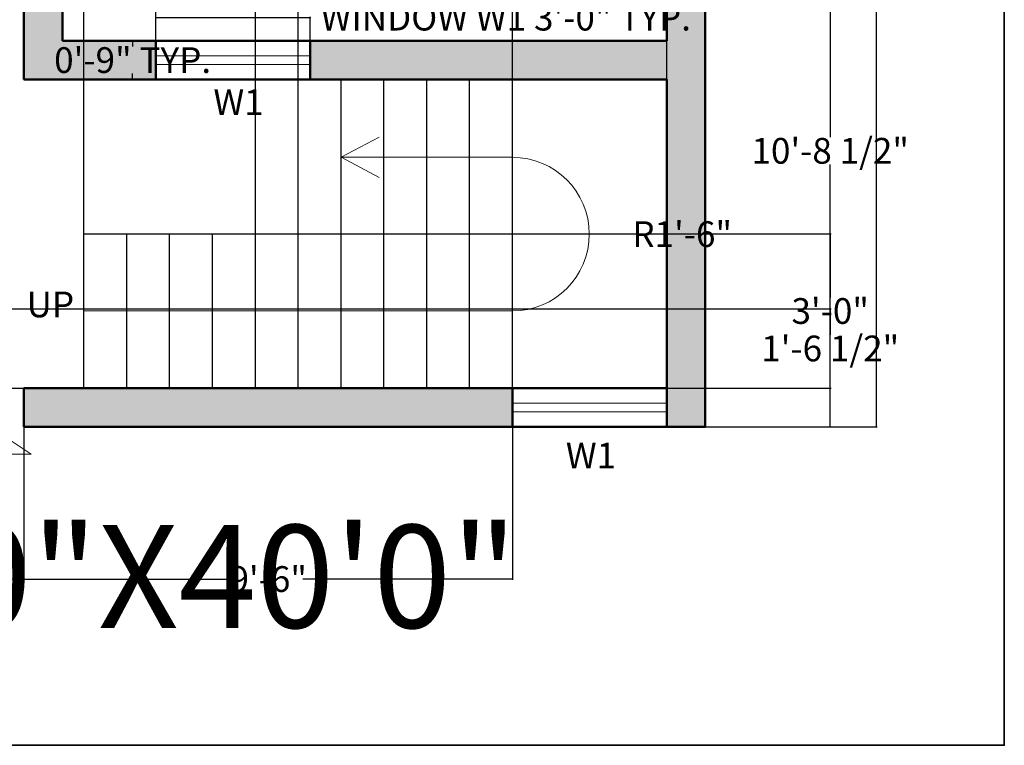
# Model space of a CAD drawing. Units: inches. Extents: x 125920 to 126336, y 366134 to 366735.
# Tile 2 of 6: x 126106 to 126336, y 366134 to 366303. Entities that reach past the tile are written whole.
import ezdxf

# ---------------------------------------------------------------- set-up
doc = ezdxf.new("R2010")
doc.units = ezdxf.units.IN
doc.header["$MEASUREMENT"] = 0
for name, color, linetype, lineweight in [('A-ANNO-DIMS', 2, 'Continuous', 18), ('A-ANNO-SYMB', 7, 'Continuous', 18), ('A-ANNO-TEXT', 7, 'Continuous', 18), ('A-ANNO-TTLB', 7, 'Continuous', 35), ('A-FLOR-STRS', 7, 'Continuous', 25), ('A-GLAZ', 4, 'Continuous', 18), ('A-WALL', 7, 'Continuous', 50)]:
    doc.layers.add(name, color=color, linetype=linetype, lineweight=lineweight)
doc.layers.add('A-WALL-PATT', color=18, linetype='Continuous', lineweight=13, true_color=0x000000)
doc.styles.get("Standard").update_dxf_attribs({"font": 'arial.ttf'})
doc.dimstyles.get("Standard").update_dxf_attribs({"dimtxt": 6, "dimasz": 0.18, "dimexe": 0.18, "dimexo": 0.0625, "dimgap": 0.09, "dimtad": 0, "dimtih": 1, "dimtoh": 1, "dimdec": 1, "dimzin": 0, "dimdsep": 46, "dimlunit": 3, "dimtxsty": 'Standard', "dimcen": 0.09, "dimadec": 0, "dimazin": 0, "dimtfac": 1, "dimtdec": 1, "dimtofl": 0, "dimtmove": 0, "dimatfit": 3, "dimfxl": 1, "dimtolj": 1, "dimtzin": 0, "dimarcsym": 0})

# ---------------------------------------------------------------- blocks, each defined once
blk = doc.blocks.new('*D4')
at = {"layer": 'A-ANNO-DIMS', "color": 0, "lineweight": -2, "transparency": 16777216}
for p, q in [((126266.54, 366688.79), (126306.57, 366688.79)), ((126306.39, 366688.61), (126306.39, 366451.45)), ((126306.39, 366207.97), (126306.39, 366445.14)), ((126266.54, 366207.79), (126306.57, 366207.79))]:
    blk.add_line(p, q, dxfattribs=at)
at = {"layer": 'A-ANNO-DIMS', "color": 0, "transparency": 16777216}
for points in [[(126306.36, 366688.61), (126306.42, 366688.61), (126306.39, 366688.79)], [(126306.36, 366207.97), (126306.42, 366207.97), (126306.39, 366207.79)]]:
    blk.add_solid(points, dxfattribs=at)
at = {"layer": 'Defpoints', "color": 0, "transparency": 16777216}
for p in [(126266.47, 366688.79), (126266.47, 366207.79), (126306.39, 366207.79)]:
    blk.add_point(p, dxfattribs=at)
at = {"layer": 'A-ANNO-DIMS', "color": 0, "transparency": 16777216, "insert": (126306.39, 366448.29), "char_height": 6, "attachment_point": 5}
blk.add_mtext('\\A1;40\'-1.0"', dxfattribs=at)
blk = doc.blocks.new('WIN-36')
for p, q in [((36, 9), (0, 9)), ((36, 5.5), (0, 5.5)), ((0, 3.5), (36, 3.5)), ((0, 0), (36, 0))]:
    blk.add_line(p, q)
blk = doc.blocks.new('*D15')
at = {"layer": 'A-ANNO-DIMS', "color": 0, "lineweight": -2, "transparency": 16777216}
for p, q in [((126138.23, 366297.86), (126138.23, 366303.37)), ((126138.41, 366303.19), (126174.05, 366303.19)), ((126174.23, 366297.86), (126174.23, 366303.37)), ((126174.23, 366303.19), (126174.41, 366303.19))]:
    blk.add_line(p, q, dxfattribs=at)
at = {"layer": 'A-ANNO-DIMS', "color": 0, "transparency": 16777216}
for points in [[(126138.41, 366303.22), (126138.41, 366303.16), (126138.23, 366303.19)], [(126174.05, 366303.22), (126174.05, 366303.16), (126174.23, 366303.19)]]:
    blk.add_solid(points, dxfattribs=at)
at = {"layer": 'Defpoints', "color": 0, "transparency": 16777216}
for p in [(126174.23, 366303.19), (126138.23, 366297.79), (126174.23, 366297.79)]:
    blk.add_point(p, dxfattribs=at)
at = {"layer": 'A-ANNO-DIMS', "color": 0, "transparency": 16777216, "insert": (126219.91, 366303.19), "char_height": 6, "attachment_point": 5}
blk.add_mtext('\\A1;WINDOW W1 3\'-0" TYP.', dxfattribs=at)
blk = doc.blocks.new('*D16')
at = {"layer": 'A-ANNO-DIMS', "color": 0, "lineweight": -2, "transparency": 16777216}
for p, q in [((126138.17, 366297.79), (126132.65, 366297.79)), ((126132.83, 366297.61), (126132.83, 366296.45)), ((126132.83, 366288.97), (126132.83, 366290.14)), ((126138.17, 366288.79), (126132.65, 366288.79))]:
    blk.add_line(p, q, dxfattribs=at)
at = {"layer": 'A-ANNO-DIMS', "color": 0, "transparency": 16777216}
for points in [[(126132.8, 366297.61), (126132.86, 366297.61), (126132.83, 366297.79)], [(126132.8, 366288.97), (126132.86, 366288.97), (126132.83, 366288.79)]]:
    blk.add_solid(points, dxfattribs=at)
at = {"layer": 'Defpoints', "color": 0, "transparency": 16777216}
for p in [(126132.83, 366297.79), (126138.23, 366297.79), (126138.23, 366288.79)]:
    blk.add_point(p, dxfattribs=at)
at = {"layer": 'A-ANNO-DIMS', "color": 0, "transparency": 16777216, "insert": (126132.83, 366293.29), "char_height": 6, "attachment_point": 5}
blk.add_mtext('\\A1;0\'-9" TYP.', dxfattribs=at)
blk = doc.blocks.new('*D32')
at = {"layer": 'A-ANNO-DIMS', "color": 0, "lineweight": -2, "transparency": 16777216}
for p, q in [((126266.54, 366336.48), (126295.8, 366336.48)), ((126295.62, 366336.3), (126295.62, 366275.33)), ((126295.62, 366207.97), (126295.62, 366268.94)), ((126266.54, 366207.79), (126295.8, 366207.79))]:
    blk.add_line(p, q, dxfattribs=at)
at = {"layer": 'A-ANNO-DIMS', "color": 0, "transparency": 16777216}
for points in [[(126295.59, 366336.3), (126295.65, 366336.3), (126295.62, 366336.48)], [(126295.59, 366207.97), (126295.65, 366207.97), (126295.62, 366207.79)]]:
    blk.add_solid(points, dxfattribs=at)
at = {"layer": 'Defpoints', "color": 0, "transparency": 16777216}
for p in [(126266.47, 366336.48), (126295.62, 366336.48), (126266.47, 366207.79)]:
    blk.add_point(p, dxfattribs=at)
at = {"layer": 'A-ANNO-DIMS', "color": 0, "transparency": 16777216, "insert": (126295.62, 366272.14), "char_height": 6, "attachment_point": 5}
blk.add_mtext('\\A1;10\'-8 1/2"', dxfattribs=at)
blk = doc.blocks.new('*D38')
at = {"layer": 'A-ANNO-DIMS', "color": 0, "lineweight": -2, "transparency": 16777216}
for p, q in [((126063.97, 366207.73), (126063.97, 366172.1)), ((126107.47, 366207.73), (126107.47, 366172.1)), ((126064.15, 366172.28), (126070.67, 366172.28)), ((126107.29, 366172.28), (126100.78, 366172.28))]:
    blk.add_line(p, q, dxfattribs=at)
at = {"layer": 'A-ANNO-DIMS', "color": 0, "transparency": 16777216}
for points in [[(126064.15, 366172.31), (126064.15, 366172.25), (126063.97, 366172.28)], [(126107.29, 366172.31), (126107.29, 366172.25), (126107.47, 366172.28)]]:
    blk.add_solid(points, dxfattribs=at)
at = {"layer": 'Defpoints', "color": 0, "transparency": 16777216}
for p in [(126063.97, 366207.79), (126107.47, 366207.79), (126107.47, 366172.28)]:
    blk.add_point(p, dxfattribs=at)
at = {"layer": 'A-ANNO-DIMS', "color": 0, "transparency": 16777216, "insert": (126085.72, 366172.28), "char_height": 6, "attachment_point": 5}
blk.add_mtext('\\A1;3\'-7 1/2"', dxfattribs=at)
blk = doc.blocks.new('*D39')
at = {"layer": 'A-ANNO-DIMS', "color": 0, "lineweight": -2, "transparency": 16777216}
for p, q in [((126107.47, 366207.73), (126107.47, 366172.1)), ((126221.47, 366207.73), (126221.47, 366172.1)), ((126107.65, 366172.28), (126156.41, 366172.28)), ((126221.29, 366172.28), (126172.54, 366172.28))]:
    blk.add_line(p, q, dxfattribs=at)
at = {"layer": 'A-ANNO-DIMS', "color": 0, "transparency": 16777216}
for points in [[(126107.65, 366172.31), (126107.65, 366172.25), (126107.47, 366172.28)], [(126221.29, 366172.31), (126221.29, 366172.25), (126221.47, 366172.28)]]:
    blk.add_solid(points, dxfattribs=at)
at = {"layer": 'Defpoints', "color": 0, "transparency": 16777216}
for p in [(126107.47, 366207.79), (126221.47, 366207.79), (126221.47, 366172.28)]:
    blk.add_point(p, dxfattribs=at)
at = {"layer": 'A-ANNO-DIMS', "color": 0, "transparency": 16777216, "insert": (126164.47, 366172.28), "char_height": 6, "attachment_point": 5}
blk.add_mtext('\\A1;9\'-6"', dxfattribs=at)
blk = doc.blocks.new('*D40')
at = {"layer": 'A-ANNO-DIMS', "color": 0, "lineweight": -2, "transparency": 16777216}
for p, q in [((126107.47, 366288.86), (126107.47, 366718.12)), ((126107.65, 366717.94), (126114.73, 366717.94)), ((126138.05, 366717.94), (126130.97, 366717.94)), ((126138.23, 366288.86), (126138.23, 366718.12))]:
    blk.add_line(p, q, dxfattribs=at)
at = {"layer": 'A-ANNO-DIMS', "color": 0, "transparency": 16777216}
for points in [[(126107.65, 366717.97), (126107.65, 366717.91), (126107.47, 366717.94)], [(126138.05, 366717.97), (126138.05, 366717.91), (126138.23, 366717.94)]]:
    blk.add_solid(points, dxfattribs=at)
at = {"layer": 'Defpoints', "color": 0, "transparency": 16777216}
for p in [(126138.23, 366717.94), (126107.47, 366288.79), (126138.23, 366288.79)]:
    blk.add_point(p, dxfattribs=at)
at = {"layer": 'A-ANNO-DIMS', "color": 0, "transparency": 16777216, "insert": (126122.85, 366717.94), "char_height": 6, "attachment_point": 5}
blk.add_mtext('\\A1;2\'-7"', dxfattribs=at)
blk = doc.blocks.new('*D41')
at = {"layer": 'A-ANNO-DIMS', "color": 0, "lineweight": -2, "transparency": 16777216}
for p, q in [((126121.47, 366216.86), (126121.47, 366718.12)), ((126121.65, 366717.94), (126163.4, 366717.94)), ((126221.29, 366717.94), (126179.54, 366717.94)), ((126221.47, 366216.86), (126221.47, 366718.12))]:
    blk.add_line(p, q, dxfattribs=at)
at = {"layer": 'A-ANNO-DIMS', "color": 0, "transparency": 16777216}
for points in [[(126121.65, 366717.97), (126121.65, 366717.91), (126121.47, 366717.94)], [(126221.29, 366717.97), (126221.29, 366717.91), (126221.47, 366717.94)]]:
    blk.add_solid(points, dxfattribs=at)
at = {"layer": 'Defpoints', "color": 0, "transparency": 16777216}
for p in [(126221.47, 366717.94), (126121.47, 366216.79), (126221.47, 366216.79)]:
    blk.add_point(p, dxfattribs=at)
at = {"layer": 'A-ANNO-DIMS', "color": 0, "transparency": 16777216, "insert": (126171.47, 366717.94), "char_height": 6, "attachment_point": 5}
blk.add_mtext('\\A1;8\'-4"', dxfattribs=at)
blk = doc.blocks.new('*D42')
at = {"layer": 'A-ANNO-DIMS', "color": 0, "lineweight": -2, "transparency": 16777216}
for p, q in [((126221.54, 366252.79), (126295.8, 366252.79)), ((126295.62, 366252.61), (126295.62, 366237.95)), ((126295.62, 366216.97), (126295.62, 366231.64)), ((126221.54, 366216.79), (126295.8, 366216.79))]:
    blk.add_line(p, q, dxfattribs=at)
at = {"layer": 'A-ANNO-DIMS', "color": 0, "transparency": 16777216}
for points in [[(126295.59, 366252.61), (126295.65, 366252.61), (126295.62, 366252.79)], [(126295.59, 366216.97), (126295.65, 366216.97), (126295.62, 366216.79)]]:
    blk.add_solid(points, dxfattribs=at)
at = {"layer": 'Defpoints', "color": 0, "transparency": 16777216}
for p in [(126221.47, 366252.79), (126295.62, 366252.79), (126221.47, 366216.79)]:
    blk.add_point(p, dxfattribs=at)
at = {"layer": 'A-ANNO-DIMS', "color": 0, "transparency": 16777216, "insert": (126295.62, 366234.79), "char_height": 6, "attachment_point": 5}
blk.add_mtext('\\A1;3\'-0"', dxfattribs=at)
blk = doc.blocks.new('*D43')
at = {"layer": 'A-ANNO-DIMS', "color": 0, "lineweight": -2, "transparency": 16777216}
for p, q in [((126221.47, 366216.86), (126221.47, 366718.12)), ((126221.65, 366717.94), (126231.41, 366717.94)), ((126257.29, 366717.94), (126247.54, 366717.94)), ((126257.47, 366216.86), (126257.47, 366718.12))]:
    blk.add_line(p, q, dxfattribs=at)
at = {"layer": 'A-ANNO-DIMS', "color": 0, "transparency": 16777216}
for points in [[(126221.65, 366717.97), (126221.65, 366717.91), (126221.47, 366717.94)], [(126257.29, 366717.97), (126257.29, 366717.91), (126257.47, 366717.94)]]:
    blk.add_solid(points, dxfattribs=at)
at = {"layer": 'Defpoints', "color": 0, "transparency": 16777216}
for p in [(126257.47, 366717.94), (126221.47, 366216.79), (126257.47, 366216.79)]:
    blk.add_point(p, dxfattribs=at)
at = {"layer": 'A-ANNO-DIMS', "color": 0, "transparency": 16777216, "insert": (126239.47, 366717.94), "char_height": 6, "attachment_point": 5}
blk.add_mtext('\\A1;3\'-0"', dxfattribs=at)
blk = doc.blocks.new('*D44')
at = {"layer": 'A-ANNO-DIMS', "color": 0, "lineweight": -2, "transparency": 16777216}
for p, q in [((126161.47, 366252.86), (126161.47, 366718.12)), ((126161.65, 366717.94), (126171.29, 366717.94)), ((126171.47, 366252.86), (126171.47, 366718.12)), ((126171.47, 366717.94), (126171.65, 366717.94))]:
    blk.add_line(p, q, dxfattribs=at)
at = {"layer": 'A-ANNO-DIMS', "color": 0, "transparency": 16777216}
for points in [[(126161.65, 366717.97), (126161.65, 366717.91), (126161.47, 366717.94)], [(126171.29, 366717.97), (126171.29, 366717.91), (126171.47, 366717.94)]]:
    blk.add_solid(points, dxfattribs=at)
at = {"layer": 'Defpoints', "color": 0, "transparency": 16777216}
for p in [(126171.47, 366717.94), (126161.47, 366252.79), (126171.47, 366252.79)]:
    blk.add_point(p, dxfattribs=at)
at = {"layer": 'A-ANNO-DIMS', "color": 0, "transparency": 16777216, "insert": (126182.05, 366717.94), "char_height": 6, "attachment_point": 5}
blk.add_mtext('\\A1;0\'-10"', dxfattribs=at)
blk = doc.blocks.new('*D46')
at = {"layer": 'A-ANNO-DIMS', "color": 0, "lineweight": -2, "transparency": 16777216}
for p, q in [((126059.54, 366235.3), (126295.8, 366235.3)), ((126295.62, 366235.12), (126295.62, 366229.24)), ((126295.62, 366216.97), (126295.62, 366222.85)), ((126059.54, 366216.79), (126295.8, 366216.79))]:
    blk.add_line(p, q, dxfattribs=at)
at = {"layer": 'A-ANNO-DIMS', "color": 0, "transparency": 16777216}
for points in [[(126295.59, 366235.12), (126295.65, 366235.12), (126295.62, 366235.3)], [(126295.59, 366216.97), (126295.65, 366216.97), (126295.62, 366216.79)]]:
    blk.add_solid(points, dxfattribs=at)
at = {"layer": 'Defpoints', "color": 0, "transparency": 16777216}
for p in [(126059.47, 366235.3), (126059.47, 366216.79), (126295.62, 366216.79)]:
    blk.add_point(p, dxfattribs=at)
at = {"layer": 'A-ANNO-DIMS', "color": 0, "transparency": 16777216, "insert": (126295.62, 366226.05), "char_height": 6, "attachment_point": 5}
blk.add_mtext('\\A1;1\'-6 1/2"', dxfattribs=at)
blk = doc.blocks.new('*D52')
at = {"layer": 'A-ANNO-DIMS', "color": 0, "lineweight": -2, "transparency": 16777216}
for p, q in [((126221.38, 366252.71), (126221.56, 366252.71)), ((126221.47, 366252.62), (126221.47, 366252.8)), ((126250.13, 366252.71), (126239.57, 366252.71))]:
    blk.add_line(p, q, dxfattribs=at)
at = {"layer": 'A-ANNO-DIMS', "color": 0, "transparency": 16777216}
blk.add_solid([(126239.57, 366252.74), (126239.57, 366252.68), (126239.39, 366252.71)], dxfattribs=at)
at = {"layer": 'Defpoints', "color": 0, "transparency": 16777216}
for p in [(126221.47, 366252.71), (126239.39, 366252.71)]:
    blk.add_point(p, dxfattribs=at)
at = {"layer": 'A-ANNO-DIMS', "color": 0, "transparency": 16777216, "insert": (126261.07, 366252.71), "char_height": 6, "attachment_point": 5}
blk.add_mtext('\\A1;R1\'-6"', dxfattribs=at)

msp = doc.modelspace()

# ---------------------------------------------------------------- hatches: boundary and pattern name
at = {"layer": 'A-WALL-PATT'}
h = msp.add_hatch(color=256, dxfattribs=at)
h.dxf.hatch_style = 1
h.paths.add_polyline_path([(126266.47, 366688.79), (125966.47, 366688.79), (125966.47, 366649.55), (125975.47, 366649.55), (125975.47, 366679.79), (126107.47, 366679.79), (126107.47, 366547.79), (126106.47, 366547.79), (126106.47, 366538.79), (126107.47, 366538.79), (126117.47, 366538.79), (126117.47, 366547.79), (126116.47, 366547.79), (126116.47, 366679.79), (126257.47, 366679.79), (126257.47, 366648.33), (126266.47, 366648.33)])
h.paths.add_polyline_path([(126070.47, 366547.79), (125975.47, 366547.79), (125975.47, 366589.55), (125966.47, 366589.55), (125966.47, 366528.42), (125975.47, 366528.42), (125975.47, 366538.79), (126059.47, 366538.79), (126059.47, 366515.79), (126063.97, 366515.79), (126063.97, 366538.79), (126070.47, 366538.79)])
h.paths.add_polyline_path([(125975.47, 366486.29), (126063.97, 366486.29), (126063.97, 366491.79), (126059.47, 366491.79), (126059.47, 366490.79), (125975.47, 366490.79), (125975.47, 366504.42), (125966.47, 366504.42), (125966.47, 366437.07), (125975.47, 366437.07)])
h.paths.add_polyline_path([(125975.47, 366312.79), (126022.47, 366312.79), (126022.47, 366317.29), (125975.47, 366317.29), (125975.47, 366377.07), (125966.47, 366377.07), (125966.47, 366207.79), (125987.64, 366207.79), (125987.64, 366216.79), (125975.47, 366216.79)])
h.paths.add_polyline_path([(126063.97, 366216.79), (126063.97, 366312.79), (126070.47, 366312.79), (126070.47, 366317.29), (126058.47, 366317.29), (126058.47, 366312.79), (126059.47, 366312.79), (126059.47, 366216.79), (126047.64, 366216.79), (126047.64, 366207.79), (126063.97, 366207.79)])
h.paths.add_polyline_path([(126221.47, 366216.79), (126116.47, 366216.79), (126107.47, 366216.79), (126107.47, 366207.79), (126221.47, 366207.79)])
h.paths.add_polyline_path([(126266.47, 366336.48), (126257.47, 366336.48), (126257.47, 366297.79), (126174.23, 366297.79), (126174.23, 366288.79), (126257.47, 366288.79), (126257.47, 366207.79), (126266.47, 366207.79)])
h.paths.add_polyline_path([(126138.23, 366297.79), (126116.47, 366297.79), (126116.47, 366433.79), (126117.47, 366433.79), (126117.47, 366438.29), (126116.47, 366438.29), (126107.47, 366438.29), (126107.47, 366317.29), (126106.47, 366317.29), (126106.47, 366312.79), (126107.47, 366312.79), (126107.47, 366288.79), (126116.47, 366288.79), (126138.23, 366288.79)])
h.paths.add_polyline_path([(126266.47, 366449.1), (126257.47, 366449.1), (126257.47, 366438.29), (126256.47, 366438.29), (126256.47, 366433.79), (126257.47, 366433.79), (126257.47, 366396.48), (126266.47, 366396.48)])
h.paths.add_polyline_path([(126232.47, 366438.29), (126180.47, 366438.29), (126180.47, 366486.29), (126257.47, 366486.29), (126257.47, 366473.1), (126266.47, 366473.1), (126266.47, 366504.78), (126257.47, 366504.78), (126257.47, 366490.79), (126180.47, 366490.79), (126180.47, 366538.79), (126232.47, 366538.79), (126232.47, 366547.79), (126153.47, 366547.79), (126153.47, 366538.79), (126175.97, 366538.79), (126175.97, 366438.29), (126153.47, 366438.29), (126153.47, 366433.79), (126232.47, 366433.79)])
h.paths.add_polyline_path([(126266.47, 366588.33), (126257.47, 366588.33), (126257.47, 366547.79), (126256.47, 366547.79), (126256.47, 366538.79), (126257.47, 366538.79), (126257.47, 366528.78), (126266.47, 366528.78)])

# ---------------------------------------------------------------- linework, layer by layer
at = {"layer": 'A-ANNO-SYMB'}
for p, q in [((126181.47, 366270.62), (126190.37, 366275.3)), ((126221.47, 366270.62), (126181.47, 366270.62)), ((126181.47, 366270.62), (126190.37, 366265.94)), ((126121.47, 366234.79), (126221.47, 366234.79)), ((126085.72, 366216.79), (126109.15, 366201.43)), ((126062.3, 366201.43), (126109.15, 366201.43))]:
    msp.add_line(p, q, dxfattribs=at)
msp.add_arc((126221.47, 366252.71), 17.91, 270, 90, dxfattribs=at)
at = {"layer": 'A-ANNO-TTLB'}
msp.add_lwpolyline([(125932.73, 366735.48), (126336.24, 366735.48), (126336.24, 366133.52), (125932.73, 366133.52)], close=True, dxfattribs=at)
at = {"layer": 'A-FLOR-STRS'}
for p, q in [((126181.47, 366216.79), (126181.47, 366288.79)), ((126191.47, 366216.79), (126191.47, 366288.79)), ((126201.47, 366216.79), (126201.47, 366288.79)), ((126211.47, 366216.79), (126211.47, 366288.79)), ((126221.47, 366216.79), (126221.47, 366288.79)), ((126121.47, 366216.79), (126121.47, 366252.79)), ((126121.47, 366252.79), (126221.47, 366252.79)), ((126131.47, 366216.79), (126131.47, 366252.79)), ((126141.47, 366216.79), (126141.47, 366252.79)), ((126151.47, 366216.79), (126151.47, 366252.79)), ((126161.47, 366216.79), (126161.47, 366252.79)), ((126171.47, 366216.79), (126171.47, 366252.79))]:
    msp.add_line(p, q, dxfattribs=at)
at = {"layer": 'A-WALL'}
for p, q in [((126266.47, 366688.79), (126266.47, 366207.79)), ((126116.47, 366433.79), (126116.47, 366297.79)), ((126257.47, 366433.79), (126257.47, 366297.79)), ((126107.47, 366312.79), (126107.47, 366288.79)), ((126116.47, 366297.79), (126257.47, 366297.79)), ((126138.23, 366297.79), (126138.23, 366288.79)), ((126174.23, 366288.79), (126174.23, 366297.79)), ((126116.47, 366288.79), (126107.47, 366288.79)), ((126116.47, 366288.79), (126257.47, 366288.79)), ((126257.47, 366288.79), (126257.47, 366207.79)), ((126107.47, 366216.79), (126107.47, 366207.79)), ((126116.47, 366216.79), (126107.47, 366216.79)), ((126116.47, 366216.79), (126257.47, 366216.79)), ((126221.47, 366216.79), (126221.47, 366207.79)), ((126107.47, 366207.79), (126266.47, 366207.79))]:
    msp.add_line(p, q, dxfattribs=at)

# ---------------------------------------------------------------- block references
at = {"layer": 'A-GLAZ'}
for p in [(126138.23, 366288.79), (126221.47, 366207.79)]:
    msp.add_blockref('WIN-36', p, dxfattribs=at)

# ---------------------------------------------------------------- texts
at = {"layer": 'A-ANNO-TEXT', "char_height": 6, "attachment_point": 1}
for s, width, insert in [('W1', 9.0002, (126151.68, 366286.48)), ('UP', 8.8759, (126108.08, 366239.32)), ('W1', 9.0002, (126233.92, 366204.09))]:
    msp.add_mtext_dynamic_manual_height_columns(s, width=width, gutter_width=30, heights=[0], dxfattribs=dict(at, insert=insert))
at = {"layer": 'A-ANNO-TTLB', "insert": (126045.63, 366184.9), "char_height": 24, "attachment_point": 1}
msp.add_mtext_dynamic_manual_height_columns('25\'0"X40\'0"', width=154.5965, gutter_width=30, heights=[0], dxfattribs=at)

# ---------------------------------------------------------------- dimensions: what is measured, and where the dimension line sits
at = {"layer": 'A-ANNO-DIMS'}
for base, p1, p2, picture, middle in [((126138.23, 366717.94), (126107.47, 366288.79), (126138.23, 366288.79), '*D40', (126122.85, 366717.94)), ((126221.47, 366717.94), (126121.47, 366216.79), (126221.47, 366216.79), '*D41', (126171.47, 366717.94)), ((126171.47, 366717.94), (126161.47, 366252.79), (126171.47, 366252.79), '*D44', (126182.05, 366717.94)), ((126257.47, 366717.94), (126221.47, 366216.79), (126257.47, 366216.79), '*D43', (126239.47, 366717.94)), ((126107.47, 366172.28), (126063.97, 366207.79), (126107.47, 366207.79), '*D38', (126085.72, 366172.28)), ((126221.47, 366172.28), (126107.47, 366207.79), (126221.47, 366207.79), '*D39', (126164.47, 366172.28))]:
    dim = msp.add_linear_dim(base=base, p1=p1, p2=p2, dimstyle='Standard', override={"dimdec": 1, "dimlfac": 1, "dimrnd": 0, "dimzin": 1, "dimdsep": 46, "dimlunit": 4, "dimfrac": 2}, dxfattribs=at)
    dim.commit()
    dim.dimension.update_dxf_attribs({"geometry": picture, "text_midpoint": middle})
for base, p1, p2, override, picture, middle in [((126306.39, 366207.79), (126266.47, 366688.79), (126266.47, 366207.79), {"dimclrd": 0, "dimclre": 0, "dimclrt": 0}, '*D4', (126306.39, 366448.29)), ((126295.62, 366336.48), (126266.47, 366207.79), (126266.47, 366336.48), {"dimdec": 1, "dimlfac": 1, "dimrnd": 0, "dimzin": 1, "dimdsep": 46, "dimlunit": 4, "dimfrac": 2}, '*D32', (126295.62, 366272.14)), ((126295.62, 366252.79), (126221.47, 366216.79), (126221.47, 366252.79), {"dimdec": 1, "dimlfac": 1, "dimrnd": 0, "dimzin": 1, "dimdsep": 46, "dimlunit": 4, "dimfrac": 2}, '*D42', (126295.62, 366234.79)), ((126295.62, 366216.79), (126059.47, 366235.3), (126059.47, 366216.79), {"dimdec": 1, "dimlfac": 1, "dimrnd": 0, "dimzin": 1, "dimdsep": 46, "dimlunit": 4, "dimfrac": 2}, '*D46', (126295.62, 366226.05))]:
    dim = msp.add_linear_dim(base=base, p1=p1, p2=p2, angle=90, dimstyle='Standard', override=override, dxfattribs=at)
    dim.commit()
    dim.dimension.update_dxf_attribs({"geometry": picture, "text_midpoint": middle})
dim = msp.add_linear_dim(base=(126174.23, 366303.19), p1=(126138.23, 366297.79), p2=(126174.23, 366297.79), text='WINDOW W1 <> TYP.', dimstyle='Standard', override={"dimdec": 1, "dimlfac": 1, "dimrnd": 0, "dimzin": 1, "dimdsep": 46, "dimlunit": 4, "dimfrac": 2}, dxfattribs=at)
dim.commit()
dim.dimension.update_dxf_attribs({"geometry": '*D15', "text_midpoint": (126219.91, 366303.19)})
dim = msp.add_linear_dim(base=(126132.83, 366297.79), p1=(126138.23, 366288.79), p2=(126138.23, 366297.79), angle=90, text='<> TYP.', dimstyle='Standard', override={"dimdec": 1, "dimlfac": 1, "dimrnd": 0, "dimzin": 1, "dimdsep": 46, "dimlunit": 4, "dimfrac": 2}, dxfattribs=at)
dim.commit()
dim.dimension.update_dxf_attribs({"geometry": '*D16', "text_midpoint": (126132.83, 366293.29)})
dim = msp.add_radius_dim(center=(126221.47, 366252.71), mpoint=(126239.39, 366252.71), dimstyle='Standard', override={"dimdec": 1, "dimlfac": 1, "dimrnd": 0, "dimzin": 1, "dimdsep": 46, "dimlunit": 4, "dimfrac": 2}, dxfattribs=at)
dim.commit()
dim.dimension.update_dxf_attribs({"geometry": '*D52', "text_midpoint": (126250.13, 366252.71), "dimtype": 164})

doc.saveas('drawing.dxf')
